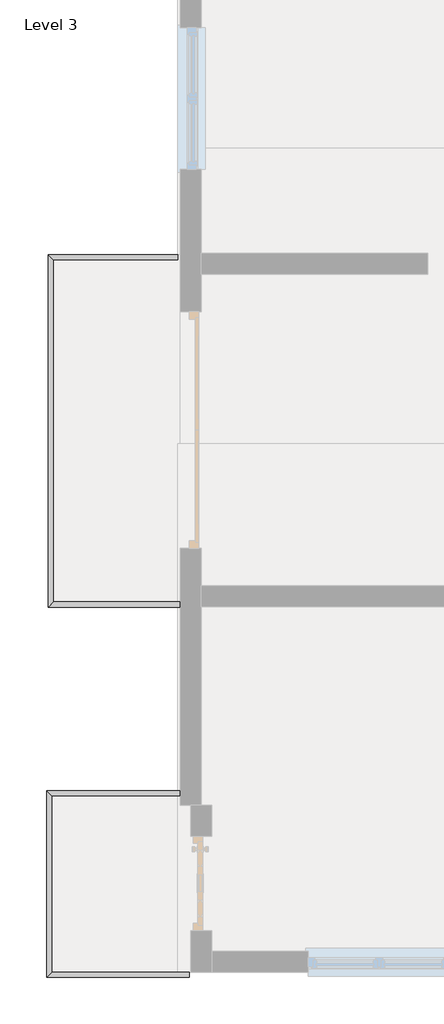
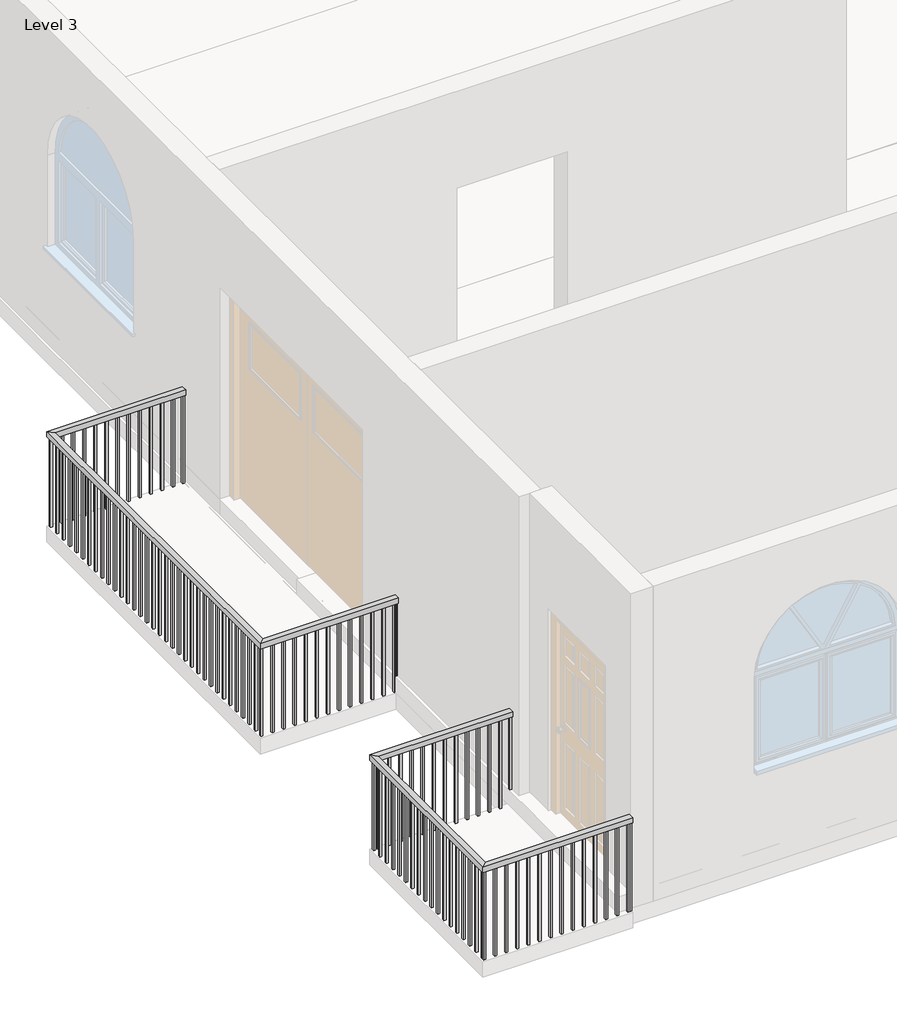
# One storey, part 3 of 7: 2 railings.
"""IFC4 building model written with IfcOpenShell, lengths in millimetres."""

from ifc_helpers import new_model, si_unit, frame, origin, place, context, project, spatial, polyline, outline, extrude, faceted_brep, element, save

model = new_model("IFC4")

# Units and contexts
model_context = context("Model", 3, world=origin())
ifc_project = project(units=[si_unit("LENGTHUNIT", "METRE", prefix="MILLI")], contexts=[model_context])

# Site, building, storey
site = spatial("IfcSite", under=ifc_project)
building = spatial("IfcBuilding", under=site)
storey = spatial("IfcBuildingStorey", under=building, Name="Level 3", Elevation=6096.0)

# Railings
placement = place(None, origin())
element("IfcRailing", 1, ObjectType="Handrail - Rectangular", at=placement, inside=storey, context=model_context, shape_type="SolidModel", body=[
    faceted_brep([(-6354.2109037, -3767.6037749, 7010.4), (-6354.2109037, -3767.6037749, 6959.6), (-6354.2109037, -3716.8037749, 6959.6), (-6354.2109037, -3716.8037749, 7010.4), (-7548.0109037, -3767.6037749, 7010.4), (-7548.0109037, -3767.6037749, 6959.6), (-7598.8109037, -3716.8037749, 6959.6), (-7598.8109037, -3716.8037749, 7010.4), (-7548.0109037, -7054.4894702, 7010.4), (-7548.0109037, -7054.4894702, 6959.6), (-7598.8109037, -7105.2894702, 6959.6), (-7598.8109037, -7105.2894702, 7010.4), (-6330.8013636, -7054.4894702, 7010.4), (-6330.8013636, -7105.2894702, 7010.4), (-6330.8013636, -7105.2894702, 6959.6), (-6330.8013636, -7054.4894702, 6959.6)], [[[0, 1, 2, 3]], [[1, 0, 4, 5]], [[2, 1, 5, 6]], [[3, 2, 6, 7]], [[0, 3, 7, 4]], [[5, 4, 8, 9]], [[6, 5, 9, 10]], [[7, 6, 10, 11]], [[4, 7, 11, 8]], [[12, 13, 14, 15]], [[9, 8, 12, 15]], [[10, 9, 15, 14]], [[11, 10, 14, 13]], [[8, 11, 13, 12]]]),
    extrude(outline(polyline([(-6363.7359037, -7089.4144702), (-6363.7359037, -7070.3644702), (-6344.6859037, -7070.3644702), (-6344.6859037, -7089.4144702), (-6363.7359037, -7089.4144702)])), frame((0.0, 0.0, 6096.0), z_axis=(0.0, 0.0, 1.0), x_axis=(1.0, 0.0, 0.0)), (0.0, 0.0, 1.0), 863.6),
    extrude(outline(polyline([(-6465.3359037, -7089.4144702), (-6465.3359037, -7070.3644702), (-6446.2859037, -7070.3644702), (-6446.2859037, -7089.4144702), (-6465.3359037, -7089.4144702)])), frame((0.0, 0.0, 6096.0), z_axis=(0.0, 0.0, 1.0), x_axis=(1.0, 0.0, 0.0)), (0.0, 0.0, 1.0), 863.6),
    extrude(outline(polyline([(-6566.9359037, -7089.4144702), (-6566.9359037, -7070.3644702), (-6547.8859037, -7070.3644702), (-6547.8859037, -7089.4144702), (-6566.9359037, -7089.4144702)])), frame((0.0, 0.0, 6096.0), z_axis=(0.0, 0.0, 1.0), x_axis=(1.0, 0.0, 0.0)), (0.0, 0.0, 1.0), 863.6),
    extrude(outline(polyline([(-6668.5359037, -7089.4144702), (-6668.5359037, -7070.3644702), (-6649.4859037, -7070.3644702), (-6649.4859037, -7089.4144702), (-6668.5359037, -7089.4144702)])), frame((0.0, 0.0, 6096.0), z_axis=(0.0, 0.0, 1.0), x_axis=(1.0, 0.0, 0.0)), (0.0, 0.0, 1.0), 863.6),
    extrude(outline(polyline([(-6770.1359037, -7089.4144702), (-6770.1359037, -7070.3644702), (-6751.0859037, -7070.3644702), (-6751.0859037, -7089.4144702), (-6770.1359037, -7089.4144702)])), frame((0.0, 0.0, 6096.0), z_axis=(0.0, 0.0, 1.0), x_axis=(1.0, 0.0, 0.0)), (0.0, 0.0, 1.0), 863.6),
    extrude(outline(polyline([(-6871.7359037, -7089.4144702), (-6871.7359037, -7070.3644702), (-6852.6859037, -7070.3644702), (-6852.6859037, -7089.4144702), (-6871.7359037, -7089.4144702)])), frame((0.0, 0.0, 6096.0), z_axis=(0.0, 0.0, 1.0), x_axis=(1.0, 0.0, 0.0)), (0.0, 0.0, 1.0), 863.6),
    extrude(outline(polyline([(-6973.3359037, -7089.4144702), (-6973.3359037, -7070.3644702), (-6954.2859037, -7070.3644702), (-6954.2859037, -7089.4144702), (-6973.3359037, -7089.4144702)])), frame((0.0, 0.0, 6096.0), z_axis=(0.0, 0.0, 1.0), x_axis=(1.0, 0.0, 0.0)), (0.0, 0.0, 1.0), 863.6),
    extrude(outline(polyline([(-7074.9359037, -7089.4144702), (-7074.9359037, -7070.3644702), (-7055.8859037, -7070.3644702), (-7055.8859037, -7089.4144702), (-7074.9359037, -7089.4144702)])), frame((0.0, 0.0, 6096.0), z_axis=(0.0, 0.0, 1.0), x_axis=(1.0, 0.0, 0.0)), (0.0, 0.0, 1.0), 863.6),
    extrude(outline(polyline([(-7176.5359037, -7089.4144702), (-7176.5359037, -7070.3644702), (-7157.4859037, -7070.3644702), (-7157.4859037, -7089.4144702), (-7176.5359037, -7089.4144702)])), frame((0.0, 0.0, 6096.0), z_axis=(0.0, 0.0, 1.0), x_axis=(1.0, 0.0, 0.0)), (0.0, 0.0, 1.0), 863.6),
    extrude(outline(polyline([(-7278.1359037, -7089.4144702), (-7278.1359037, -7070.3644702), (-7259.0859037, -7070.3644702), (-7259.0859037, -7089.4144702), (-7278.1359037, -7089.4144702)])), frame((0.0, 0.0, 6096.0), z_axis=(0.0, 0.0, 1.0), x_axis=(1.0, 0.0, 0.0)), (0.0, 0.0, 1.0), 863.6),
    extrude(outline(polyline([(-7379.7359037, -7089.4144702), (-7379.7359037, -7070.3644702), (-7360.6859037, -7070.3644702), (-7360.6859037, -7089.4144702), (-7379.7359037, -7089.4144702)])), frame((0.0, 0.0, 6096.0), z_axis=(0.0, 0.0, 1.0), x_axis=(1.0, 0.0, 0.0)), (0.0, 0.0, 1.0), 863.6),
    extrude(outline(polyline([(-7481.3359037, -7089.4144702), (-7481.3359037, -7070.3644702), (-7462.2859037, -7070.3644702), (-7462.2859037, -7089.4144702), (-7481.3359037, -7089.4144702)])), frame((0.0, 0.0, 6096.0), z_axis=(0.0, 0.0, 1.0), x_axis=(1.0, 0.0, 0.0)), (0.0, 0.0, 1.0), 863.6),
    extrude(outline(polyline([(-7582.9359037, -6983.8787749), (-7563.8859037, -6983.8787749), (-7563.8859037, -7002.9287749), (-7582.9359037, -7002.9287749), (-7582.9359037, -6983.8787749)])), frame((0.0, 0.0, 6096.0), z_axis=(0.0, 0.0, 1.0), x_axis=(1.0, 0.0, 0.0)), (0.0, 0.0, 1.0), 863.6),
    extrude(outline(polyline([(-7582.9359037, -6882.2787749), (-7563.8859037, -6882.2787749), (-7563.8859037, -6901.3287749), (-7582.9359037, -6901.3287749), (-7582.9359037, -6882.2787749)])), frame((0.0, 0.0, 6096.0), z_axis=(0.0, 0.0, 1.0), x_axis=(1.0, 0.0, 0.0)), (0.0, 0.0, 1.0), 863.6),
    extrude(outline(polyline([(-7582.9359037, -6780.6787749), (-7563.8859037, -6780.6787749), (-7563.8859037, -6799.7287749), (-7582.9359037, -6799.7287749), (-7582.9359037, -6780.6787749)])), frame((0.0, 0.0, 6096.0), z_axis=(0.0, 0.0, 1.0), x_axis=(1.0, 0.0, 0.0)), (0.0, 0.0, 1.0), 863.6),
    extrude(outline(polyline([(-7582.9359037, -6679.0787749), (-7563.8859037, -6679.0787749), (-7563.8859037, -6698.1287749), (-7582.9359037, -6698.1287749), (-7582.9359037, -6679.0787749)])), frame((0.0, 0.0, 6096.0), z_axis=(0.0, 0.0, 1.0), x_axis=(1.0, 0.0, 0.0)), (0.0, 0.0, 1.0), 863.6),
    extrude(outline(polyline([(-7582.9359037, -6577.4787749), (-7563.8859037, -6577.4787749), (-7563.8859037, -6596.5287749), (-7582.9359037, -6596.5287749), (-7582.9359037, -6577.4787749)])), frame((0.0, 0.0, 6096.0), z_axis=(0.0, 0.0, 1.0), x_axis=(1.0, 0.0, 0.0)), (0.0, 0.0, 1.0), 863.6),
    extrude(outline(polyline([(-7582.9359037, -6475.8787749), (-7563.8859037, -6475.8787749), (-7563.8859037, -6494.9287749), (-7582.9359037, -6494.9287749), (-7582.9359037, -6475.8787749)])), frame((0.0, 0.0, 6096.0), z_axis=(0.0, 0.0, 1.0), x_axis=(1.0, 0.0, 0.0)), (0.0, 0.0, 1.0), 863.6),
    extrude(outline(polyline([(-7582.9359037, -6374.2787749), (-7563.8859037, -6374.2787749), (-7563.8859037, -6393.3287749), (-7582.9359037, -6393.3287749), (-7582.9359037, -6374.2787749)])), frame((0.0, 0.0, 6096.0), z_axis=(0.0, 0.0, 1.0), x_axis=(1.0, 0.0, 0.0)), (0.0, 0.0, 1.0), 863.6),
    extrude(outline(polyline([(-7582.9359037, -6272.6787749), (-7563.8859037, -6272.6787749), (-7563.8859037, -6291.7287749), (-7582.9359037, -6291.7287749), (-7582.9359037, -6272.6787749)])), frame((0.0, 0.0, 6096.0), z_axis=(0.0, 0.0, 1.0), x_axis=(1.0, 0.0, 0.0)), (0.0, 0.0, 1.0), 863.6),
    extrude(outline(polyline([(-7582.9359037, -6171.0787749), (-7563.8859037, -6171.0787749), (-7563.8859037, -6190.1287749), (-7582.9359037, -6190.1287749), (-7582.9359037, -6171.0787749)])), frame((0.0, 0.0, 6096.0), z_axis=(0.0, 0.0, 1.0), x_axis=(1.0, 0.0, 0.0)), (0.0, 0.0, 1.0), 863.6),
    extrude(outline(polyline([(-7582.9359037, -6069.4787749), (-7563.8859037, -6069.4787749), (-7563.8859037, -6088.5287749), (-7582.9359037, -6088.5287749), (-7582.9359037, -6069.4787749)])), frame((0.0, 0.0, 6096.0), z_axis=(0.0, 0.0, 1.0), x_axis=(1.0, 0.0, 0.0)), (0.0, 0.0, 1.0), 863.6),
    extrude(outline(polyline([(-7582.9359037, -5967.8787749), (-7563.8859037, -5967.8787749), (-7563.8859037, -5986.9287749), (-7582.9359037, -5986.9287749), (-7582.9359037, -5967.8787749)])), frame((0.0, 0.0, 6096.0), z_axis=(0.0, 0.0, 1.0), x_axis=(1.0, 0.0, 0.0)), (0.0, 0.0, 1.0), 863.6),
    extrude(outline(polyline([(-7582.9359037, -5866.2787749), (-7563.8859037, -5866.2787749), (-7563.8859037, -5885.3287749), (-7582.9359037, -5885.3287749), (-7582.9359037, -5866.2787749)])), frame((0.0, 0.0, 6096.0), z_axis=(0.0, 0.0, 1.0), x_axis=(1.0, 0.0, 0.0)), (0.0, 0.0, 1.0), 863.6),
    extrude(outline(polyline([(-7582.9359037, -5764.6787749), (-7563.8859037, -5764.6787749), (-7563.8859037, -5783.7287749), (-7582.9359037, -5783.7287749), (-7582.9359037, -5764.6787749)])), frame((0.0, 0.0, 6096.0), z_axis=(0.0, 0.0, 1.0), x_axis=(1.0, 0.0, 0.0)), (0.0, 0.0, 1.0), 863.6),
    extrude(outline(polyline([(-7582.9359037, -5663.0787749), (-7563.8859037, -5663.0787749), (-7563.8859037, -5682.1287749), (-7582.9359037, -5682.1287749), (-7582.9359037, -5663.0787749)])), frame((0.0, 0.0, 6096.0), z_axis=(0.0, 0.0, 1.0), x_axis=(1.0, 0.0, 0.0)), (0.0, 0.0, 1.0), 863.6),
    extrude(outline(polyline([(-7582.9359037, -5561.4787749), (-7563.8859037, -5561.4787749), (-7563.8859037, -5580.5287749), (-7582.9359037, -5580.5287749), (-7582.9359037, -5561.4787749)])), frame((0.0, 0.0, 6096.0), z_axis=(0.0, 0.0, 1.0), x_axis=(1.0, 0.0, 0.0)), (0.0, 0.0, 1.0), 863.6),
    extrude(outline(polyline([(-7582.9359037, -5459.8787749), (-7563.8859037, -5459.8787749), (-7563.8859037, -5478.9287749), (-7582.9359037, -5478.9287749), (-7582.9359037, -5459.8787749)])), frame((0.0, 0.0, 6096.0), z_axis=(0.0, 0.0, 1.0), x_axis=(1.0, 0.0, 0.0)), (0.0, 0.0, 1.0), 863.6),
    extrude(outline(polyline([(-7582.9359037, -5358.2787749), (-7563.8859037, -5358.2787749), (-7563.8859037, -5377.3287749), (-7582.9359037, -5377.3287749), (-7582.9359037, -5358.2787749)])), frame((0.0, 0.0, 6096.0), z_axis=(0.0, 0.0, 1.0), x_axis=(1.0, 0.0, 0.0)), (0.0, 0.0, 1.0), 863.6),
    extrude(outline(polyline([(-7582.9359037, -5256.6787749), (-7563.8859037, -5256.6787749), (-7563.8859037, -5275.7287749), (-7582.9359037, -5275.7287749), (-7582.9359037, -5256.6787749)])), frame((0.0, 0.0, 6096.0), z_axis=(0.0, 0.0, 1.0), x_axis=(1.0, 0.0, 0.0)), (0.0, 0.0, 1.0), 863.6),
    extrude(outline(polyline([(-7582.9359037, -5155.0787749), (-7563.8859037, -5155.0787749), (-7563.8859037, -5174.1287749), (-7582.9359037, -5174.1287749), (-7582.9359037, -5155.0787749)])), frame((0.0, 0.0, 6096.0), z_axis=(0.0, 0.0, 1.0), x_axis=(1.0, 0.0, 0.0)), (0.0, 0.0, 1.0), 863.6),
    extrude(outline(polyline([(-7582.9359037, -5053.4787749), (-7563.8859037, -5053.4787749), (-7563.8859037, -5072.5287749), (-7582.9359037, -5072.5287749), (-7582.9359037, -5053.4787749)])), frame((0.0, 0.0, 6096.0), z_axis=(0.0, 0.0, 1.0), x_axis=(1.0, 0.0, 0.0)), (0.0, 0.0, 1.0), 863.6),
    extrude(outline(polyline([(-7582.9359037, -4951.8787749), (-7563.8859037, -4951.8787749), (-7563.8859037, -4970.9287749), (-7582.9359037, -4970.9287749), (-7582.9359037, -4951.8787749)])), frame((0.0, 0.0, 6096.0), z_axis=(0.0, 0.0, 1.0), x_axis=(1.0, 0.0, 0.0)), (0.0, 0.0, 1.0), 863.6),
    extrude(outline(polyline([(-7582.9359037, -4850.2787749), (-7563.8859037, -4850.2787749), (-7563.8859037, -4869.3287749), (-7582.9359037, -4869.3287749), (-7582.9359037, -4850.2787749)])), frame((0.0, 0.0, 6096.0), z_axis=(0.0, 0.0, 1.0), x_axis=(1.0, 0.0, 0.0)), (0.0, 0.0, 1.0), 863.6),
    extrude(outline(polyline([(-7582.9359037, -4748.6787749), (-7563.8859037, -4748.6787749), (-7563.8859037, -4767.7287749), (-7582.9359037, -4767.7287749), (-7582.9359037, -4748.6787749)])), frame((0.0, 0.0, 6096.0), z_axis=(0.0, 0.0, 1.0), x_axis=(1.0, 0.0, 0.0)), (0.0, 0.0, 1.0), 863.6),
    extrude(outline(polyline([(-7582.9359037, -4647.0787749), (-7563.8859037, -4647.0787749), (-7563.8859037, -4666.1287749), (-7582.9359037, -4666.1287749), (-7582.9359037, -4647.0787749)])), frame((0.0, 0.0, 6096.0), z_axis=(0.0, 0.0, 1.0), x_axis=(1.0, 0.0, 0.0)), (0.0, 0.0, 1.0), 863.6),
    extrude(outline(polyline([(-7582.9359037, -4545.4787749), (-7563.8859037, -4545.4787749), (-7563.8859037, -4564.5287749), (-7582.9359037, -4564.5287749), (-7582.9359037, -4545.4787749)])), frame((0.0, 0.0, 6096.0), z_axis=(0.0, 0.0, 1.0), x_axis=(1.0, 0.0, 0.0)), (0.0, 0.0, 1.0), 863.6),
    extrude(outline(polyline([(-7582.9359037, -4443.8787749), (-7563.8859037, -4443.8787749), (-7563.8859037, -4462.9287749), (-7582.9359037, -4462.9287749), (-7582.9359037, -4443.8787749)])), frame((0.0, 0.0, 6096.0), z_axis=(0.0, 0.0, 1.0), x_axis=(1.0, 0.0, 0.0)), (0.0, 0.0, 1.0), 863.6),
    extrude(outline(polyline([(-7582.9359037, -4342.2787749), (-7563.8859037, -4342.2787749), (-7563.8859037, -4361.3287749), (-7582.9359037, -4361.3287749), (-7582.9359037, -4342.2787749)])), frame((0.0, 0.0, 6096.0), z_axis=(0.0, 0.0, 1.0), x_axis=(1.0, 0.0, 0.0)), (0.0, 0.0, 1.0), 863.6),
    extrude(outline(polyline([(-7582.9359037, -4240.6787749), (-7563.8859037, -4240.6787749), (-7563.8859037, -4259.7287749), (-7582.9359037, -4259.7287749), (-7582.9359037, -4240.6787749)])), frame((0.0, 0.0, 6096.0), z_axis=(0.0, 0.0, 1.0), x_axis=(1.0, 0.0, 0.0)), (0.0, 0.0, 1.0), 863.6),
    extrude(outline(polyline([(-7582.9359037, -4139.0787749), (-7563.8859037, -4139.0787749), (-7563.8859037, -4158.1287749), (-7582.9359037, -4158.1287749), (-7582.9359037, -4139.0787749)])), frame((0.0, 0.0, 6096.0), z_axis=(0.0, 0.0, 1.0), x_axis=(1.0, 0.0, 0.0)), (0.0, 0.0, 1.0), 863.6),
    extrude(outline(polyline([(-7582.9359037, -4037.4787749), (-7563.8859037, -4037.4787749), (-7563.8859037, -4056.5287749), (-7582.9359037, -4056.5287749), (-7582.9359037, -4037.4787749)])), frame((0.0, 0.0, 6096.0), z_axis=(0.0, 0.0, 1.0), x_axis=(1.0, 0.0, 0.0)), (0.0, 0.0, 1.0), 863.6),
    extrude(outline(polyline([(-7582.9359037, -3935.8787749), (-7563.8859037, -3935.8787749), (-7563.8859037, -3954.9287749), (-7582.9359037, -3954.9287749), (-7582.9359037, -3935.8787749)])), frame((0.0, 0.0, 6096.0), z_axis=(0.0, 0.0, 1.0), x_axis=(1.0, 0.0, 0.0)), (0.0, 0.0, 1.0), 863.6),
    extrude(outline(polyline([(-7582.9359037, -3834.2787749), (-7563.8859037, -3834.2787749), (-7563.8859037, -3853.3287749), (-7582.9359037, -3853.3287749), (-7582.9359037, -3834.2787749)])), frame((0.0, 0.0, 6096.0), z_axis=(0.0, 0.0, 1.0), x_axis=(1.0, 0.0, 0.0)), (0.0, 0.0, 1.0), 863.6),
    extrude(outline(polyline([(-7462.2859037, -3732.6787749), (-7462.2859037, -3751.7287749), (-7481.3359037, -3751.7287749), (-7481.3359037, -3732.6787749), (-7462.2859037, -3732.6787749)])), frame((0.0, 0.0, 6096.0), z_axis=(0.0, 0.0, 1.0), x_axis=(1.0, 0.0, 0.0)), (0.0, 0.0, 1.0), 863.6),
    extrude(outline(polyline([(-7360.6859037, -3732.6787749), (-7360.6859037, -3751.7287749), (-7379.7359037, -3751.7287749), (-7379.7359037, -3732.6787749), (-7360.6859037, -3732.6787749)])), frame((0.0, 0.0, 6096.0), z_axis=(0.0, 0.0, 1.0), x_axis=(1.0, 0.0, 0.0)), (0.0, 0.0, 1.0), 863.6),
    extrude(outline(polyline([(-7259.0859037, -3732.6787749), (-7259.0859037, -3751.7287749), (-7278.1359037, -3751.7287749), (-7278.1359037, -3732.6787749), (-7259.0859037, -3732.6787749)])), frame((0.0, 0.0, 6096.0), z_axis=(0.0, 0.0, 1.0), x_axis=(1.0, 0.0, 0.0)), (0.0, 0.0, 1.0), 863.6),
    extrude(outline(polyline([(-7157.4859037, -3732.6787749), (-7157.4859037, -3751.7287749), (-7176.5359037, -3751.7287749), (-7176.5359037, -3732.6787749), (-7157.4859037, -3732.6787749)])), frame((0.0, 0.0, 6096.0), z_axis=(0.0, 0.0, 1.0), x_axis=(1.0, 0.0, 0.0)), (0.0, 0.0, 1.0), 863.6),
    extrude(outline(polyline([(-7055.8859037, -3732.6787749), (-7055.8859037, -3751.7287749), (-7074.9359037, -3751.7287749), (-7074.9359037, -3732.6787749), (-7055.8859037, -3732.6787749)])), frame((0.0, 0.0, 6096.0), z_axis=(0.0, 0.0, 1.0), x_axis=(1.0, 0.0, 0.0)), (0.0, 0.0, 1.0), 863.6),
    extrude(outline(polyline([(-6954.2859037, -3732.6787749), (-6954.2859037, -3751.7287749), (-6973.3359037, -3751.7287749), (-6973.3359037, -3732.6787749), (-6954.2859037, -3732.6787749)])), frame((0.0, 0.0, 6096.0), z_axis=(0.0, 0.0, 1.0), x_axis=(1.0, 0.0, 0.0)), (0.0, 0.0, 1.0), 863.6),
    extrude(outline(polyline([(-6852.6859037, -3732.6787749), (-6852.6859037, -3751.7287749), (-6871.7359037, -3751.7287749), (-6871.7359037, -3732.6787749), (-6852.6859037, -3732.6787749)])), frame((0.0, 0.0, 6096.0), z_axis=(0.0, 0.0, 1.0), x_axis=(1.0, 0.0, 0.0)), (0.0, 0.0, 1.0), 863.6),
    extrude(outline(polyline([(-6751.0859037, -3732.6787749), (-6751.0859037, -3751.7287749), (-6770.1359037, -3751.7287749), (-6770.1359037, -3732.6787749), (-6751.0859037, -3732.6787749)])), frame((0.0, 0.0, 6096.0), z_axis=(0.0, 0.0, 1.0), x_axis=(1.0, 0.0, 0.0)), (0.0, 0.0, 1.0), 863.6),
    extrude(outline(polyline([(-6649.4859037, -3732.6787749), (-6649.4859037, -3751.7287749), (-6668.5359037, -3751.7287749), (-6668.5359037, -3732.6787749), (-6649.4859037, -3732.6787749)])), frame((0.0, 0.0, 6096.0), z_axis=(0.0, 0.0, 1.0), x_axis=(1.0, 0.0, 0.0)), (0.0, 0.0, 1.0), 863.6),
    extrude(outline(polyline([(-6547.8859037, -3732.6787749), (-6547.8859037, -3751.7287749), (-6566.9359037, -3751.7287749), (-6566.9359037, -3732.6787749), (-6547.8859037, -3732.6787749)])), frame((0.0, 0.0, 6096.0), z_axis=(0.0, 0.0, 1.0), x_axis=(1.0, 0.0, 0.0)), (0.0, 0.0, 1.0), 863.6),
    extrude(outline(polyline([(-6446.2859037, -3732.6787749), (-6446.2859037, -3751.7287749), (-6465.3359037, -3751.7287749), (-6465.3359037, -3732.6787749), (-6446.2859037, -3732.6787749)])), frame((0.0, 0.0, 6096.0), z_axis=(0.0, 0.0, 1.0), x_axis=(1.0, 0.0, 0.0)), (0.0, 0.0, 1.0), 863.6),
    extrude(outline(polyline([(-7582.9359037, -7070.3644702), (-7563.8859037, -7070.3644702), (-7563.8859037, -7089.4144702), (-7582.9359037, -7089.4144702), (-7582.9359037, -7070.3644702)])), frame((0.0, 0.0, 6096.0), z_axis=(0.0, 0.0, 1.0), x_axis=(1.0, 0.0, 0.0)), (0.0, 0.0, 1.0), 863.6),
    extrude(outline(polyline([(-7563.8859037, -3732.6787749), (-7563.8859037, -3751.7287749), (-7582.9359037, -3751.7287749), (-7582.9359037, -3732.6787749), (-7563.8859037, -3732.6787749)])), frame((0.0, 0.0, 6096.0), z_axis=(0.0, 0.0, 1.0), x_axis=(1.0, 0.0, 0.0)), (0.0, 0.0, 1.0), 863.6),
    extrude(outline(polyline([(-6349.8513636, -7089.4144702), (-6349.8513636, -7070.3644702), (-6330.8013636, -7070.3644702), (-6330.8013636, -7089.4144702), (-6349.8513636, -7089.4144702)])), frame((0.0, 0.0, 6096.0), z_axis=(0.0, 0.0, 1.0), x_axis=(1.0, 0.0, 0.0)), (0.0, 0.0, 1.0), 863.6),
    extrude(outline(polyline([(-6354.2109037, -3732.6787749), (-6354.2109037, -3751.7287749), (-6373.2609037, -3751.7287749), (-6373.2609037, -3732.6787749), (-6354.2109037, -3732.6787749)])), frame((0.0, 0.0, 6096.0), z_axis=(0.0, 0.0, 1.0), x_axis=(1.0, 0.0, 0.0)), (0.0, 0.0, 1.0), 863.6),
])
element("IfcRailing", 2, ObjectType="Handrail - Rectangular", at=placement, inside=storey, context=model_context, shape_type="SolidModel", body=[
    faceted_brep([(-6330.8013636, -8918.8845215, 7010.4), (-6330.8013636, -8918.8845215, 6959.6), (-6330.8013636, -8868.0845215, 6959.6), (-6330.8013636, -8868.0845215, 7010.4), (-7563.8859037, -8918.8845215, 7010.4), (-7563.8859037, -8918.8845215, 6959.6), (-7614.6859037, -8868.0845215, 6959.6), (-7614.6859037, -8868.0845215, 7010.4), (-7563.8859037, -10612.9037749, 7010.4), (-7563.8859037, -10612.9037749, 6959.6), (-7614.6859037, -10663.7037749, 6959.6), (-7614.6859037, -10663.7037749, 7010.4), (-6243.0859037, -10612.9037749, 7010.4), (-6243.0859037, -10663.7037749, 7010.4), (-6243.0859037, -10663.7037749, 6959.6), (-6243.0859037, -10612.9037749, 6959.6)], [[[0, 1, 2, 3]], [[1, 0, 4, 5]], [[2, 1, 5, 6]], [[3, 2, 6, 7]], [[0, 3, 7, 4]], [[5, 4, 8, 9]], [[6, 5, 9, 10]], [[7, 6, 10, 11]], [[4, 7, 11, 8]], [[12, 13, 14, 15]], [[9, 8, 12, 15]], [[10, 9, 15, 14]], [[11, 10, 14, 13]], [[8, 11, 13, 12]]]),
    extrude(outline(polyline([(-6278.0109037, -10647.8287749), (-6278.0109037, -10628.7787749), (-6258.9609037, -10628.7787749), (-6258.9609037, -10647.8287749), (-6278.0109037, -10647.8287749)])), frame((0.0, 0.0, 6096.0), z_axis=(0.0, 0.0, 1.0), x_axis=(1.0, 0.0, 0.0)), (0.0, 0.0, 1.0), 863.6),
    extrude(outline(polyline([(-6379.6109037, -10647.8287749), (-6379.6109037, -10628.7787749), (-6360.5609037, -10628.7787749), (-6360.5609037, -10647.8287749), (-6379.6109037, -10647.8287749)])), frame((0.0, 0.0, 6096.0), z_axis=(0.0, 0.0, 1.0), x_axis=(1.0, 0.0, 0.0)), (0.0, 0.0, 1.0), 863.6),
    extrude(outline(polyline([(-6481.2109037, -10647.8287749), (-6481.2109037, -10628.7787749), (-6462.1609037, -10628.7787749), (-6462.1609037, -10647.8287749), (-6481.2109037, -10647.8287749)])), frame((0.0, 0.0, 6096.0), z_axis=(0.0, 0.0, 1.0), x_axis=(1.0, 0.0, 0.0)), (0.0, 0.0, 1.0), 863.6),
    extrude(outline(polyline([(-6582.8109037, -10647.8287749), (-6582.8109037, -10628.7787749), (-6563.7609037, -10628.7787749), (-6563.7609037, -10647.8287749), (-6582.8109037, -10647.8287749)])), frame((0.0, 0.0, 6096.0), z_axis=(0.0, 0.0, 1.0), x_axis=(1.0, 0.0, 0.0)), (0.0, 0.0, 1.0), 863.6),
    extrude(outline(polyline([(-6684.4109037, -10647.8287749), (-6684.4109037, -10628.7787749), (-6665.3609037, -10628.7787749), (-6665.3609037, -10647.8287749), (-6684.4109037, -10647.8287749)])), frame((0.0, 0.0, 6096.0), z_axis=(0.0, 0.0, 1.0), x_axis=(1.0, 0.0, 0.0)), (0.0, 0.0, 1.0), 863.6),
    extrude(outline(polyline([(-6786.0109037, -10647.8287749), (-6786.0109037, -10628.7787749), (-6766.9609037, -10628.7787749), (-6766.9609037, -10647.8287749), (-6786.0109037, -10647.8287749)])), frame((0.0, 0.0, 6096.0), z_axis=(0.0, 0.0, 1.0), x_axis=(1.0, 0.0, 0.0)), (0.0, 0.0, 1.0), 863.6),
    extrude(outline(polyline([(-6887.6109037, -10647.8287749), (-6887.6109037, -10628.7787749), (-6868.5609037, -10628.7787749), (-6868.5609037, -10647.8287749), (-6887.6109037, -10647.8287749)])), frame((0.0, 0.0, 6096.0), z_axis=(0.0, 0.0, 1.0), x_axis=(1.0, 0.0, 0.0)), (0.0, 0.0, 1.0), 863.6),
    extrude(outline(polyline([(-6989.2109037, -10647.8287749), (-6989.2109037, -10628.7787749), (-6970.1609037, -10628.7787749), (-6970.1609037, -10647.8287749), (-6989.2109037, -10647.8287749)])), frame((0.0, 0.0, 6096.0), z_axis=(0.0, 0.0, 1.0), x_axis=(1.0, 0.0, 0.0)), (0.0, 0.0, 1.0), 863.6),
    extrude(outline(polyline([(-7090.8109037, -10647.8287749), (-7090.8109037, -10628.7787749), (-7071.7609037, -10628.7787749), (-7071.7609037, -10647.8287749), (-7090.8109037, -10647.8287749)])), frame((0.0, 0.0, 6096.0), z_axis=(0.0, 0.0, 1.0), x_axis=(1.0, 0.0, 0.0)), (0.0, 0.0, 1.0), 863.6),
    extrude(outline(polyline([(-7192.4109037, -10647.8287749), (-7192.4109037, -10628.7787749), (-7173.3609037, -10628.7787749), (-7173.3609037, -10647.8287749), (-7192.4109037, -10647.8287749)])), frame((0.0, 0.0, 6096.0), z_axis=(0.0, 0.0, 1.0), x_axis=(1.0, 0.0, 0.0)), (0.0, 0.0, 1.0), 863.6),
    extrude(outline(polyline([(-7294.0109037, -10647.8287749), (-7294.0109037, -10628.7787749), (-7274.9609037, -10628.7787749), (-7274.9609037, -10647.8287749), (-7294.0109037, -10647.8287749)])), frame((0.0, 0.0, 6096.0), z_axis=(0.0, 0.0, 1.0), x_axis=(1.0, 0.0, 0.0)), (0.0, 0.0, 1.0), 863.6),
    extrude(outline(polyline([(-7395.6109037, -10647.8287749), (-7395.6109037, -10628.7787749), (-7376.5609037, -10628.7787749), (-7376.5609037, -10647.8287749), (-7395.6109037, -10647.8287749)])), frame((0.0, 0.0, 6096.0), z_axis=(0.0, 0.0, 1.0), x_axis=(1.0, 0.0, 0.0)), (0.0, 0.0, 1.0), 863.6),
    extrude(outline(polyline([(-7497.2109037, -10647.8287749), (-7497.2109037, -10628.7787749), (-7478.1609037, -10628.7787749), (-7478.1609037, -10647.8287749), (-7497.2109037, -10647.8287749)])), frame((0.0, 0.0, 6096.0), z_axis=(0.0, 0.0, 1.0), x_axis=(1.0, 0.0, 0.0)), (0.0, 0.0, 1.0), 863.6),
    extrude(outline(polyline([(-7598.8109037, -10611.1595215), (-7579.7609037, -10611.1595215), (-7579.7609037, -10630.2095215), (-7598.8109037, -10630.2095215), (-7598.8109037, -10611.1595215)])), frame((0.0, 0.0, 6096.0), z_axis=(0.0, 0.0, 1.0), x_axis=(1.0, 0.0, 0.0)), (0.0, 0.0, 1.0), 863.6),
    extrude(outline(polyline([(-7598.8109037, -10509.5595215), (-7579.7609037, -10509.5595215), (-7579.7609037, -10528.6095215), (-7598.8109037, -10528.6095215), (-7598.8109037, -10509.5595215)])), frame((0.0, 0.0, 6096.0), z_axis=(0.0, 0.0, 1.0), x_axis=(1.0, 0.0, 0.0)), (0.0, 0.0, 1.0), 863.6),
    extrude(outline(polyline([(-7598.8109037, -10407.9595215), (-7579.7609037, -10407.9595215), (-7579.7609037, -10427.0095215), (-7598.8109037, -10427.0095215), (-7598.8109037, -10407.9595215)])), frame((0.0, 0.0, 6096.0), z_axis=(0.0, 0.0, 1.0), x_axis=(1.0, 0.0, 0.0)), (0.0, 0.0, 1.0), 863.6),
    extrude(outline(polyline([(-7598.8109037, -10306.3595215), (-7579.7609037, -10306.3595215), (-7579.7609037, -10325.4095215), (-7598.8109037, -10325.4095215), (-7598.8109037, -10306.3595215)])), frame((0.0, 0.0, 6096.0), z_axis=(0.0, 0.0, 1.0), x_axis=(1.0, 0.0, 0.0)), (0.0, 0.0, 1.0), 863.6),
    extrude(outline(polyline([(-7598.8109037, -10204.7595215), (-7579.7609037, -10204.7595215), (-7579.7609037, -10223.8095215), (-7598.8109037, -10223.8095215), (-7598.8109037, -10204.7595215)])), frame((0.0, 0.0, 6096.0), z_axis=(0.0, 0.0, 1.0), x_axis=(1.0, 0.0, 0.0)), (0.0, 0.0, 1.0), 863.6),
    extrude(outline(polyline([(-7598.8109037, -10103.1595215), (-7579.7609037, -10103.1595215), (-7579.7609037, -10122.2095215), (-7598.8109037, -10122.2095215), (-7598.8109037, -10103.1595215)])), frame((0.0, 0.0, 6096.0), z_axis=(0.0, 0.0, 1.0), x_axis=(1.0, 0.0, 0.0)), (0.0, 0.0, 1.0), 863.6),
    extrude(outline(polyline([(-7598.8109037, -10001.5595215), (-7579.7609037, -10001.5595215), (-7579.7609037, -10020.6095215), (-7598.8109037, -10020.6095215), (-7598.8109037, -10001.5595215)])), frame((0.0, 0.0, 6096.0), z_axis=(0.0, 0.0, 1.0), x_axis=(1.0, 0.0, 0.0)), (0.0, 0.0, 1.0), 863.6),
    extrude(outline(polyline([(-7598.8109037, -9899.9595215), (-7579.7609037, -9899.9595215), (-7579.7609037, -9919.0095215), (-7598.8109037, -9919.0095215), (-7598.8109037, -9899.9595215)])), frame((0.0, 0.0, 6096.0), z_axis=(0.0, 0.0, 1.0), x_axis=(1.0, 0.0, 0.0)), (0.0, 0.0, 1.0), 863.6),
    extrude(outline(polyline([(-7598.8109037, -9798.3595215), (-7579.7609037, -9798.3595215), (-7579.7609037, -9817.4095215), (-7598.8109037, -9817.4095215), (-7598.8109037, -9798.3595215)])), frame((0.0, 0.0, 6096.0), z_axis=(0.0, 0.0, 1.0), x_axis=(1.0, 0.0, 0.0)), (0.0, 0.0, 1.0), 863.6),
    extrude(outline(polyline([(-7598.8109037, -9696.7595215), (-7579.7609037, -9696.7595215), (-7579.7609037, -9715.8095215), (-7598.8109037, -9715.8095215), (-7598.8109037, -9696.7595215)])), frame((0.0, 0.0, 6096.0), z_axis=(0.0, 0.0, 1.0), x_axis=(1.0, 0.0, 0.0)), (0.0, 0.0, 1.0), 863.6),
    extrude(outline(polyline([(-7598.8109037, -9595.1595215), (-7579.7609037, -9595.1595215), (-7579.7609037, -9614.2095215), (-7598.8109037, -9614.2095215), (-7598.8109037, -9595.1595215)])), frame((0.0, 0.0, 6096.0), z_axis=(0.0, 0.0, 1.0), x_axis=(1.0, 0.0, 0.0)), (0.0, 0.0, 1.0), 863.6),
    extrude(outline(polyline([(-7598.8109037, -9493.5595215), (-7579.7609037, -9493.5595215), (-7579.7609037, -9512.6095215), (-7598.8109037, -9512.6095215), (-7598.8109037, -9493.5595215)])), frame((0.0, 0.0, 6096.0), z_axis=(0.0, 0.0, 1.0), x_axis=(1.0, 0.0, 0.0)), (0.0, 0.0, 1.0), 863.6),
    extrude(outline(polyline([(-7598.8109037, -9391.9595215), (-7579.7609037, -9391.9595215), (-7579.7609037, -9411.0095215), (-7598.8109037, -9411.0095215), (-7598.8109037, -9391.9595215)])), frame((0.0, 0.0, 6096.0), z_axis=(0.0, 0.0, 1.0), x_axis=(1.0, 0.0, 0.0)), (0.0, 0.0, 1.0), 863.6),
    extrude(outline(polyline([(-7598.8109037, -9290.3595215), (-7579.7609037, -9290.3595215), (-7579.7609037, -9309.4095215), (-7598.8109037, -9309.4095215), (-7598.8109037, -9290.3595215)])), frame((0.0, 0.0, 6096.0), z_axis=(0.0, 0.0, 1.0), x_axis=(1.0, 0.0, 0.0)), (0.0, 0.0, 1.0), 863.6),
    extrude(outline(polyline([(-7598.8109037, -9188.7595215), (-7579.7609037, -9188.7595215), (-7579.7609037, -9207.8095215), (-7598.8109037, -9207.8095215), (-7598.8109037, -9188.7595215)])), frame((0.0, 0.0, 6096.0), z_axis=(0.0, 0.0, 1.0), x_axis=(1.0, 0.0, 0.0)), (0.0, 0.0, 1.0), 863.6),
    extrude(outline(polyline([(-7598.8109037, -9087.1595215), (-7579.7609037, -9087.1595215), (-7579.7609037, -9106.2095215), (-7598.8109037, -9106.2095215), (-7598.8109037, -9087.1595215)])), frame((0.0, 0.0, 6096.0), z_axis=(0.0, 0.0, 1.0), x_axis=(1.0, 0.0, 0.0)), (0.0, 0.0, 1.0), 863.6),
    extrude(outline(polyline([(-7598.8109037, -8985.5595215), (-7579.7609037, -8985.5595215), (-7579.7609037, -9004.6095215), (-7598.8109037, -9004.6095215), (-7598.8109037, -8985.5595215)])), frame((0.0, 0.0, 6096.0), z_axis=(0.0, 0.0, 1.0), x_axis=(1.0, 0.0, 0.0)), (0.0, 0.0, 1.0), 863.6),
    extrude(outline(polyline([(-7540.4763636, -8883.9595215), (-7540.4763636, -8903.0095215), (-7559.5263636, -8903.0095215), (-7559.5263636, -8883.9595215), (-7540.4763636, -8883.9595215)])), frame((0.0, 0.0, 6096.0), z_axis=(0.0, 0.0, 1.0), x_axis=(1.0, 0.0, 0.0)), (0.0, 0.0, 1.0), 863.6),
    extrude(outline(polyline([(-7438.8763636, -8883.9595215), (-7438.8763636, -8903.0095215), (-7457.9263636, -8903.0095215), (-7457.9263636, -8883.9595215), (-7438.8763636, -8883.9595215)])), frame((0.0, 0.0, 6096.0), z_axis=(0.0, 0.0, 1.0), x_axis=(1.0, 0.0, 0.0)), (0.0, 0.0, 1.0), 863.6),
    extrude(outline(polyline([(-7337.2763636, -8883.9595215), (-7337.2763636, -8903.0095215), (-7356.3263636, -8903.0095215), (-7356.3263636, -8883.9595215), (-7337.2763636, -8883.9595215)])), frame((0.0, 0.0, 6096.0), z_axis=(0.0, 0.0, 1.0), x_axis=(1.0, 0.0, 0.0)), (0.0, 0.0, 1.0), 863.6),
    extrude(outline(polyline([(-7235.6763636, -8883.9595215), (-7235.6763636, -8903.0095215), (-7254.7263636, -8903.0095215), (-7254.7263636, -8883.9595215), (-7235.6763636, -8883.9595215)])), frame((0.0, 0.0, 6096.0), z_axis=(0.0, 0.0, 1.0), x_axis=(1.0, 0.0, 0.0)), (0.0, 0.0, 1.0), 863.6),
    extrude(outline(polyline([(-7134.0763636, -8883.9595215), (-7134.0763636, -8903.0095215), (-7153.1263636, -8903.0095215), (-7153.1263636, -8883.9595215), (-7134.0763636, -8883.9595215)])), frame((0.0, 0.0, 6096.0), z_axis=(0.0, 0.0, 1.0), x_axis=(1.0, 0.0, 0.0)), (0.0, 0.0, 1.0), 863.6),
    extrude(outline(polyline([(-7032.4763636, -8883.9595215), (-7032.4763636, -8903.0095215), (-7051.5263636, -8903.0095215), (-7051.5263636, -8883.9595215), (-7032.4763636, -8883.9595215)])), frame((0.0, 0.0, 6096.0), z_axis=(0.0, 0.0, 1.0), x_axis=(1.0, 0.0, 0.0)), (0.0, 0.0, 1.0), 863.6),
    extrude(outline(polyline([(-6930.8763636, -8883.9595215), (-6930.8763636, -8903.0095215), (-6949.9263636, -8903.0095215), (-6949.9263636, -8883.9595215), (-6930.8763636, -8883.9595215)])), frame((0.0, 0.0, 6096.0), z_axis=(0.0, 0.0, 1.0), x_axis=(1.0, 0.0, 0.0)), (0.0, 0.0, 1.0), 863.6),
    extrude(outline(polyline([(-6829.2763636, -8883.9595215), (-6829.2763636, -8903.0095215), (-6848.3263636, -8903.0095215), (-6848.3263636, -8883.9595215), (-6829.2763636, -8883.9595215)])), frame((0.0, 0.0, 6096.0), z_axis=(0.0, 0.0, 1.0), x_axis=(1.0, 0.0, 0.0)), (0.0, 0.0, 1.0), 863.6),
    extrude(outline(polyline([(-6727.6763636, -8883.9595215), (-6727.6763636, -8903.0095215), (-6746.7263636, -8903.0095215), (-6746.7263636, -8883.9595215), (-6727.6763636, -8883.9595215)])), frame((0.0, 0.0, 6096.0), z_axis=(0.0, 0.0, 1.0), x_axis=(1.0, 0.0, 0.0)), (0.0, 0.0, 1.0), 863.6),
    extrude(outline(polyline([(-6626.0763636, -8883.9595215), (-6626.0763636, -8903.0095215), (-6645.1263636, -8903.0095215), (-6645.1263636, -8883.9595215), (-6626.0763636, -8883.9595215)])), frame((0.0, 0.0, 6096.0), z_axis=(0.0, 0.0, 1.0), x_axis=(1.0, 0.0, 0.0)), (0.0, 0.0, 1.0), 863.6),
    extrude(outline(polyline([(-6524.4763636, -8883.9595215), (-6524.4763636, -8903.0095215), (-6543.5263636, -8903.0095215), (-6543.5263636, -8883.9595215), (-6524.4763636, -8883.9595215)])), frame((0.0, 0.0, 6096.0), z_axis=(0.0, 0.0, 1.0), x_axis=(1.0, 0.0, 0.0)), (0.0, 0.0, 1.0), 863.6),
    extrude(outline(polyline([(-6422.8763636, -8883.9595215), (-6422.8763636, -8903.0095215), (-6441.9263636, -8903.0095215), (-6441.9263636, -8883.9595215), (-6422.8763636, -8883.9595215)])), frame((0.0, 0.0, 6096.0), z_axis=(0.0, 0.0, 1.0), x_axis=(1.0, 0.0, 0.0)), (0.0, 0.0, 1.0), 863.6),
    extrude(outline(polyline([(-7598.8109037, -10628.7787749), (-7579.7609037, -10628.7787749), (-7579.7609037, -10647.8287749), (-7598.8109037, -10647.8287749), (-7598.8109037, -10628.7787749)])), frame((0.0, 0.0, 6096.0), z_axis=(0.0, 0.0, 1.0), x_axis=(1.0, 0.0, 0.0)), (0.0, 0.0, 1.0), 863.6),
    extrude(outline(polyline([(-7579.7609037, -8883.9595215), (-7579.7609037, -8903.0095215), (-7598.8109037, -8903.0095215), (-7598.8109037, -8883.9595215), (-7579.7609037, -8883.9595215)])), frame((0.0, 0.0, 6096.0), z_axis=(0.0, 0.0, 1.0), x_axis=(1.0, 0.0, 0.0)), (0.0, 0.0, 1.0), 863.6),
    extrude(outline(polyline([(-6262.1359037, -10647.8287749), (-6262.1359037, -10628.7787749), (-6243.0859037, -10628.7787749), (-6243.0859037, -10647.8287749), (-6262.1359037, -10647.8287749)])), frame((0.0, 0.0, 6096.0), z_axis=(0.0, 0.0, 1.0), x_axis=(1.0, 0.0, 0.0)), (0.0, 0.0, 1.0), 863.6),
    extrude(outline(polyline([(-6330.8013636, -8883.9595215), (-6330.8013636, -8903.0095215), (-6349.8513636, -8903.0095215), (-6349.8513636, -8883.9595215), (-6330.8013636, -8883.9595215)])), frame((0.0, 0.0, 6096.0), z_axis=(0.0, 0.0, 1.0), x_axis=(1.0, 0.0, 0.0)), (0.0, 0.0, 1.0), 863.6),
])

save(model, "model.ifc")

# Revit data of these elements
# Type "Handrail - Rectangular"
#   Assembly Code = "C2010400"
#   built-in parameter 1008612 = 0.0416667 (stored number, unit not read)
#   built-in parameter 1008611 = 0.0416667 (stored number, unit not read)
#   built-in parameter 1008609 = 0.333333 (stored number, unit not read)
#   built-in parameter 1008604 = 0.166667 (stored number, unit not read)
#   built-in parameter 1008603 = 0.166667 (stored number, unit not read)
#   Railing Height = 3' - 0"
#   built-in parameter 1008630 = 2
#   built-in parameter 1008610 = 2
#   built-in parameter 1008618 = Baluster - Square : 3/4"
# Elements 1, 2 (IfcRailing, "Handrail - Rectangular")
#   Phase Created = New Construction
